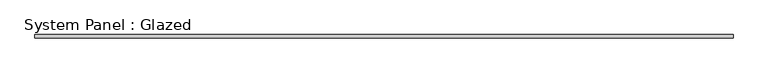
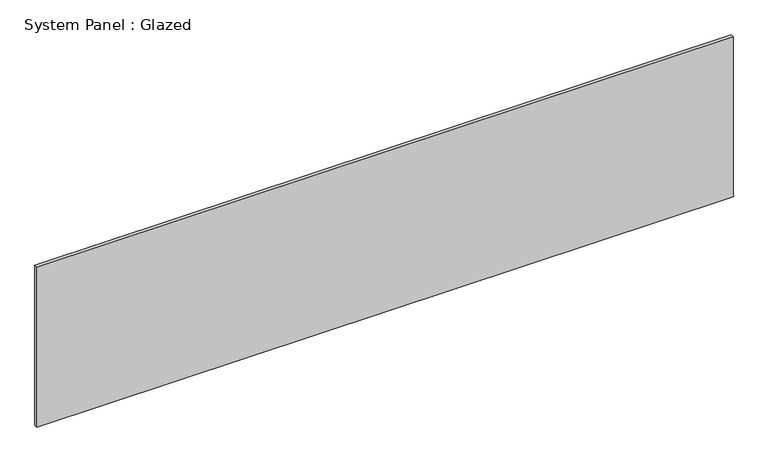
"""IFC4 building model written with IfcOpenShell, lengths in millimetres: plate geometry, System Panel : Glazed."""

from ifc_helpers import new_model, si_unit, origin, origin_with_axes, place, context, project, spatial, polyline, outline, extrude, source, transform, mapped, element, save


def system_panel_glazed_c55d8a5b(model_context):
    return source(origin(), model_context, "Body", "SweptSolid", [
        extrude(outline(polyline([(2514.6, 19.05), (-2514.6, 19.05), (-2514.6, 44.45), (2514.6, 44.45), (2514.6, 19.05)])), origin_with_axes(), (0.0, 0.0, 1.0), 1219.2),
    ])


if __name__ == "__main__":
    model = new_model("IFC4")
    model_context = context("Model", 3, world=origin())
    ifc_project = project(units=[si_unit("LENGTHUNIT", "METRE", prefix="MILLI")], contexts=[model_context])
    site = spatial("IfcSite", under=ifc_project)
    building = spatial("IfcBuilding", under=site)
    placement = place(None, origin())
    system_panel_glazed_shape = system_panel_glazed_c55d8a5b(model_context)
    element("IfcPlate", 1, ObjectType="System Panel : Glazed", at=placement, inside=building, context=model_context, shape_type="MappedRepresentation", body=[
        mapped(system_panel_glazed_shape, transform((0.0, 0.0, 0.0), x_axis=(1.0, 0.0, 0.0), y_axis=(0.0, 1.0, 0.0), z_axis=(0.0, 0.0, 1.0))),
    ])
    save(model, "model.ifc")

# Revit data of these elements
# Type "System Panel : Glazed"
#   Construction Type Id = "GSP4R"
#   Analytic Construction = "1/8 in Pilkington single glazing"
#   Visual Light Transmittance = 0.9
#   Solar Heat Gain Coefficient = 0.86
#   Heat Transfer Coefficient (U) = 1.18115 BTU/(h·ft²·°F)
# Element 1 (IfcPlate, "System Panel : Glazed")
#   Materials on its faces: "Glass"
# Materials
#   "Glass": class "Glass", colour RGB 0 128 192, transparency 0.75, Description = "Soda Lime Glass", Cost = 0
